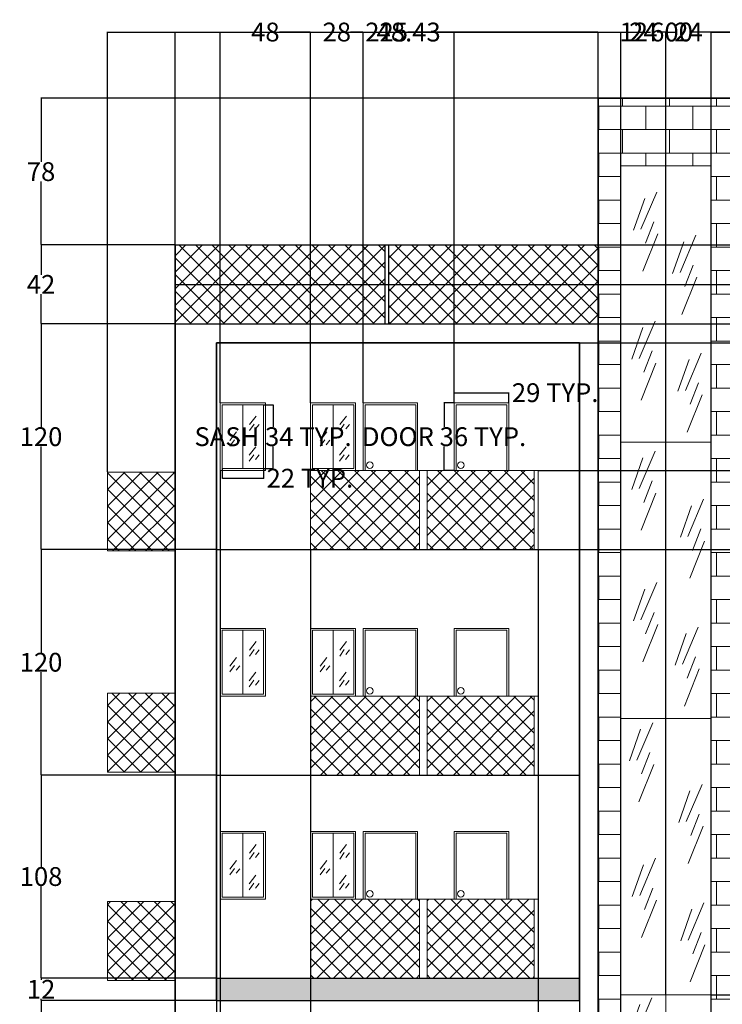
# Model space of a CAD drawing. Units: inches. Extents: x 183 to 891, y 196 to 984.
# Tile 2 of 3: x 192 to 566, y 460 to 984. Entities that reach past the tile are written whole.
import ezdxf

# ---------------------------------------------------------------- set-up
doc = ezdxf.new("R2010")
doc.units = ezdxf.units.IN
doc.header["$MEASUREMENT"] = 0
for name, color, linetype, lineweight in [('A-ANNO-DIMS', 2, 'Continuous', 18), ('A-DOOR', 3, 'Continuous', 20), ('A-FLOR', 7, 'Continuous', 30), ('A-FLOR-PATT', 2, 'Continuous', 13), ('A-GLAZ', 4, 'Continuous', 18), ('A-GLAZ-DETL', 4, 'Continuous', 13), ('A-RAIL', 7, 'Continuous', 20), ('A-RAIL-PATT', 8, 'Continuous', 13), ('A-ROOF', 7, 'Continuous', 25), ('A-WALL', 7, 'Continuous', 35), ('A-WALL-PATT', 251, 'Continuous', 13)]:
    doc.layers.add(name, color=color, linetype=linetype, lineweight=lineweight)
doc.styles.get("Standard").update_dxf_attribs({"font": 'arial.ttf'})
doc.dimstyles.get("Standard").update_dxf_attribs({"dimtxt": 10, "dimasz": 0.18, "dimexe": 0.18, "dimexo": 0.0625, "dimgap": 0.09, "dimtad": 0, "dimtih": 1, "dimtoh": 1, "dimdec": 0, "dimzin": 0, "dimdsep": 46, "dimlunit": 3, "dimtxsty": 'Standard', "dimcen": 0.09, "dimadec": 0, "dimazin": 0, "dimtfac": 1, "dimtdec": 0, "dimtofl": 0, "dimtmove": 0, "dimatfit": 3, "dimfxl": 1, "dimtolj": 1, "dimtzin": 0, "dimarcsym": 0})

# ---------------------------------------------------------------- blocks, each defined once
blk = doc.blocks.new('WIN-SASH-PAIR-22X34')
for p, q in [((11, 34), (11, 0)), ((18.11, 27.96), (14.53, 23.4)), ((16.98, 23.73), (14.53, 20.31)), ((19.74, 23.56), (17.79, 21.12)), ((7.74, 19.54), (4.16, 14.99)), ((6.61, 15.31), (4.16, 11.9)), ((9.37, 15.15), (7.42, 12.71)), ((18.01, 11.64), (14.43, 7.09)), ((16.87, 7.41), (14.43, 4)), ((19.64, 7.25), (17.69, 4.81))]:
    blk.add_line(p, q)
blk.add_lwpolyline([(0, 0), (22, 0), (22, 34), (0, 34)], close=True)
blk = doc.blocks.new('DOOR-BALCONY-ELEV-29')
for p, q in [((0, 0), (0, 36)), ((0, 36), (29, 36)), ((1, 35), (28, 35)), ((1, 0), (1, 35)), ((28, 35), (28, 0)), ((29, 36), (29, 0))]:
    blk.add_line(p, q)
blk.add_circle((3.53, 2.84), 1.74)
blk = doc.blocks.new('GLASS-REFLECTION-ELEV')
for p, q in [((12.39, 42.09), (3.96, 22.28)), ((5.95, 38.63), (0, 21.79)), ((10.9, 26.25), (6.44, 14.86)), ((12.89, 19.81), (4.96, 0))]:
    blk.add_line(p, q)
blk = doc.blocks.new('*D4')
at = {"layer": 'A-ANNO-DIMS', "color": 0, "lineweight": -2, "transparency": 16777216}
for p, q in [((321.66, 778.68), (326.88, 778.68)), ((326.7, 778.5), (326.7, 766.94)), ((326.7, 744.86), (326.7, 756.41)), ((321.66, 744.68), (326.88, 744.68))]:
    blk.add_line(p, q, dxfattribs=at)
at = {"layer": 'A-ANNO-DIMS', "color": 0, "transparency": 16777216}
for points in [[(326.67, 778.5), (326.73, 778.5), (326.7, 778.68)], [(326.67, 744.86), (326.73, 744.86), (326.7, 744.68)]]:
    blk.add_solid(points, dxfattribs=at)
at = {"layer": 'Defpoints', "color": 0, "transparency": 16777216}
for p in [(321.6, 778.68), (326.7, 778.68), (321.6, 744.68)]:
    blk.add_point(p, dxfattribs=at)
at = {"layer": 'A-ANNO-DIMS', "color": 0, "transparency": 16777216, "insert": (326.7, 761.68), "char_height": 10, "attachment_point": 5}
blk.add_mtext('\\A1;SASH 34 TYP.', dxfattribs=at)
blk = doc.blocks.new('*D5')
at = {"layer": 'A-ANNO-DIMS', "color": 0, "lineweight": -2, "transparency": 16777216}
for p, q in [((299.6, 744.61), (299.6, 739.4)), ((321.6, 744.61), (321.6, 739.4)), ((299.78, 739.58), (321.42, 739.58)), ((321.6, 739.58), (321.78, 739.58))]:
    blk.add_line(p, q, dxfattribs=at)
at = {"layer": 'A-ANNO-DIMS', "color": 0, "transparency": 16777216}
for points in [[(299.78, 739.61), (299.78, 739.55), (299.6, 739.58)], [(321.42, 739.61), (321.42, 739.55), (321.6, 739.58)]]:
    blk.add_solid(points, dxfattribs=at)
at = {"layer": 'Defpoints', "color": 0, "transparency": 16777216}
for p in [(299.6, 744.68), (321.6, 744.68), (321.6, 739.58)]:
    blk.add_point(p, dxfattribs=at)
at = {"layer": 'A-ANNO-DIMS', "color": 0, "transparency": 16777216, "insert": (346.29, 739.58), "char_height": 10, "attachment_point": 5}
blk.add_mtext('\\A1;22 TYP.', dxfattribs=at)
blk = doc.blocks.new('*D6')
at = {"layer": 'A-ANNO-DIMS', "color": 0, "lineweight": -2, "transparency": 16777216}
for p, q in [((422.96, 779.68), (417.45, 779.68)), ((417.63, 779.5), (417.63, 766.94)), ((417.63, 743.86), (417.63, 756.41)), ((422.96, 743.68), (417.45, 743.68))]:
    blk.add_line(p, q, dxfattribs=at)
at = {"layer": 'A-ANNO-DIMS', "color": 0, "transparency": 16777216}
for points in [[(417.6, 779.5), (417.66, 779.5), (417.63, 779.68)], [(417.6, 743.86), (417.66, 743.86), (417.63, 743.68)]]:
    blk.add_solid(points, dxfattribs=at)
at = {"layer": 'Defpoints', "color": 0, "transparency": 16777216}
for p in [(417.63, 779.68), (423.03, 779.68), (423.03, 743.68)]:
    blk.add_point(p, dxfattribs=at)
at = {"layer": 'A-ANNO-DIMS', "color": 0, "transparency": 16777216, "insert": (417.63, 761.68), "char_height": 10, "attachment_point": 5}
blk.add_mtext('\\A1;DOOR 36 TYP.', dxfattribs=at)
blk = doc.blocks.new('*D7')
at = {"layer": 'A-ANNO-DIMS', "color": 0, "lineweight": -2, "transparency": 16777216}
for p, q in [((423.03, 779.74), (423.03, 785.26)), ((423.21, 785.08), (451.85, 785.08)), ((452.03, 779.74), (452.03, 785.26)), ((452.03, 785.08), (452.21, 785.08))]:
    blk.add_line(p, q, dxfattribs=at)
at = {"layer": 'A-ANNO-DIMS', "color": 0, "transparency": 16777216}
for points in [[(423.21, 785.11), (423.21, 785.05), (423.03, 785.08)], [(451.85, 785.11), (451.85, 785.05), (452.03, 785.08)]]:
    blk.add_solid(points, dxfattribs=at)
at = {"layer": 'Defpoints', "color": 0, "transparency": 16777216}
for p in [(452.03, 785.08), (423.03, 779.68), (452.03, 779.68)]:
    blk.add_point(p, dxfattribs=at)
at = {"layer": 'A-ANNO-DIMS', "color": 0, "transparency": 16777216, "insert": (476.72, 785.08), "char_height": 10, "attachment_point": 5}
blk.add_mtext('\\A1;29 TYP.', dxfattribs=at)
blk = doc.blocks.new('*D8')
at = {"layer": 'A-ANNO-DIMS', "color": 0, "lineweight": -2, "transparency": 16777216}
for p, q in [((238.6, 742.93), (238.6, 977.12)), ((238.78, 976.94), (527.45, 976.94)), ((838.42, 976.94), (549.75, 976.94)), ((838.6, 743.74), (838.6, 977.12))]:
    blk.add_line(p, q, dxfattribs=at)
at = {"layer": 'A-ANNO-DIMS', "color": 0, "transparency": 16777216}
for points in [[(238.78, 976.97), (238.78, 976.91), (238.6, 976.94)], [(838.42, 976.97), (838.42, 976.91), (838.6, 976.94)]]:
    blk.add_solid(points, dxfattribs=at)
at = {"layer": 'Defpoints', "color": 0, "transparency": 16777216}
for p in [(838.6, 976.94), (238.6, 742.86), (838.6, 743.68)]:
    blk.add_point(p, dxfattribs=at)
at = {"layer": 'A-ANNO-DIMS', "color": 0, "transparency": 16777216, "insert": (538.6, 976.94), "char_height": 10, "attachment_point": 5}
blk.add_mtext('\\A1;600', dxfattribs=at)
blk = doc.blocks.new('*D10')
at = {"layer": 'A-ANNO-DIMS', "color": 0, "lineweight": -2, "transparency": 16777216}
for p, q in [((274.6, 863.74), (274.6, 977.12)), ((274.78, 976.94), (375.84, 976.94)), ((499.42, 976.94), (398.36, 976.94)), ((499.6, 863.74), (499.6, 977.12))]:
    blk.add_line(p, q, dxfattribs=at)
at = {"layer": 'A-ANNO-DIMS', "color": 0, "transparency": 16777216}
for points in [[(274.78, 976.97), (274.78, 976.91), (274.6, 976.94)], [(499.42, 976.97), (499.42, 976.91), (499.6, 976.94)]]:
    blk.add_solid(points, dxfattribs=at)
at = {"layer": 'Defpoints', "color": 0, "transparency": 16777216}
for p in [(499.6, 976.94), (274.6, 863.68), (499.6, 863.68)]:
    blk.add_point(p, dxfattribs=at)
at = {"layer": 'A-ANNO-DIMS', "color": 0, "transparency": 16777216, "insert": (387.1, 976.94), "char_height": 10, "attachment_point": 5}
blk.add_mtext('\\A1;225', dxfattribs=at)
blk = doc.blocks.new('*D27')
at = {"layer": 'A-ANNO-DIMS', "color": 0, "lineweight": -2, "transparency": 16777216}
for p, q in [((296.54, 461.68), (203.15, 461.68)), ((203.33, 461.5), (203.33, 406.87)), ((203.33, 341.86), (203.33, 396.48)), ((274.54, 341.68), (203.15, 341.68))]:
    blk.add_line(p, q, dxfattribs=at)
at = {"layer": 'A-ANNO-DIMS', "color": 0, "transparency": 16777216}
for points in [[(203.3, 461.5), (203.36, 461.5), (203.33, 461.68)], [(203.3, 341.86), (203.36, 341.86), (203.33, 341.68)]]:
    blk.add_solid(points, dxfattribs=at)
at = {"layer": 'Defpoints', "color": 0, "transparency": 16777216}
for p in [(203.33, 461.68), (296.6, 461.68), (274.6, 341.68)]:
    blk.add_point(p, dxfattribs=at)
at = {"layer": 'A-ANNO-DIMS', "color": 0, "transparency": 16777216, "insert": (203.33, 401.68), "char_height": 10, "attachment_point": 5}
blk.add_mtext('\\A1;120', dxfattribs=at)
blk = doc.blocks.new('*D28')
at = {"layer": 'A-ANNO-DIMS', "color": 0, "lineweight": -2, "transparency": 16777216}
for p, q in [((296.54, 473.68), (203.15, 473.68)), ((203.33, 473.5), (203.33, 472.79)), ((296.54, 461.68), (203.15, 461.68)), ((203.33, 461.86), (203.33, 462.56))]:
    blk.add_line(p, q, dxfattribs=at)
at = {"layer": 'A-ANNO-DIMS', "color": 0, "transparency": 16777216}
for points in [[(203.3, 473.5), (203.36, 473.5), (203.33, 473.68)], [(203.3, 461.86), (203.36, 461.86), (203.33, 461.68)]]:
    blk.add_solid(points, dxfattribs=at)
at = {"layer": 'Defpoints', "color": 0, "transparency": 16777216}
for p in [(203.33, 473.68), (296.6, 473.68), (296.6, 461.68)]:
    blk.add_point(p, dxfattribs=at)
at = {"layer": 'A-ANNO-DIMS', "color": 0, "transparency": 16777216, "insert": (203.33, 467.68), "char_height": 10, "attachment_point": 5}
blk.add_mtext('\\A1;12', dxfattribs=at)
blk = doc.blocks.new('*D29')
at = {"layer": 'A-ANNO-DIMS', "color": 0, "lineweight": -2, "transparency": 16777216}
for p, q in [((296.54, 581.68), (203.15, 581.68)), ((203.33, 581.5), (203.33, 532.87)), ((203.33, 473.86), (203.33, 522.48)), ((296.54, 473.68), (203.15, 473.68))]:
    blk.add_line(p, q, dxfattribs=at)
at = {"layer": 'A-ANNO-DIMS', "color": 0, "transparency": 16777216}
for points in [[(203.3, 581.5), (203.36, 581.5), (203.33, 581.68)], [(203.3, 473.86), (203.36, 473.86), (203.33, 473.68)]]:
    blk.add_solid(points, dxfattribs=at)
at = {"layer": 'Defpoints', "color": 0, "transparency": 16777216}
for p in [(203.33, 581.68), (296.6, 581.68), (296.6, 473.68)]:
    blk.add_point(p, dxfattribs=at)
at = {"layer": 'A-ANNO-DIMS', "color": 0, "transparency": 16777216, "insert": (203.33, 527.68), "char_height": 10, "attachment_point": 5}
blk.add_mtext('\\A1;108', dxfattribs=at)
blk = doc.blocks.new('*D30')
at = {"layer": 'A-ANNO-DIMS', "color": 0, "lineweight": -2, "transparency": 16777216}
for p, q in [((296.54, 701.68), (203.15, 701.68)), ((203.33, 701.5), (203.33, 646.87)), ((203.33, 581.86), (203.33, 636.48)), ((296.54, 581.68), (203.15, 581.68))]:
    blk.add_line(p, q, dxfattribs=at)
at = {"layer": 'A-ANNO-DIMS', "color": 0, "transparency": 16777216}
for points in [[(203.3, 701.5), (203.36, 701.5), (203.33, 701.68)], [(203.3, 581.86), (203.36, 581.86), (203.33, 581.68)]]:
    blk.add_solid(points, dxfattribs=at)
at = {"layer": 'Defpoints', "color": 0, "transparency": 16777216}
for p in [(203.33, 701.68), (296.6, 701.68), (296.6, 581.68)]:
    blk.add_point(p, dxfattribs=at)
at = {"layer": 'A-ANNO-DIMS', "color": 0, "transparency": 16777216, "insert": (203.33, 641.68), "char_height": 10, "attachment_point": 5}
blk.add_mtext('\\A1;120', dxfattribs=at)
blk = doc.blocks.new('*D31')
at = {"layer": 'A-ANNO-DIMS', "color": 0, "lineweight": -2, "transparency": 16777216}
for p, q in [((274.54, 821.68), (203.15, 821.68)), ((203.33, 821.5), (203.33, 766.87)), ((203.33, 701.86), (203.33, 756.48)), ((296.54, 701.68), (203.15, 701.68))]:
    blk.add_line(p, q, dxfattribs=at)
at = {"layer": 'A-ANNO-DIMS', "color": 0, "transparency": 16777216}
for points in [[(203.3, 821.5), (203.36, 821.5), (203.33, 821.68)], [(203.3, 701.86), (203.36, 701.86), (203.33, 701.68)]]:
    blk.add_solid(points, dxfattribs=at)
at = {"layer": 'Defpoints', "color": 0, "transparency": 16777216}
for p in [(203.33, 821.68), (274.6, 821.68), (296.6, 701.68)]:
    blk.add_point(p, dxfattribs=at)
at = {"layer": 'A-ANNO-DIMS', "color": 0, "transparency": 16777216, "insert": (203.33, 761.68), "char_height": 10, "attachment_point": 5}
blk.add_mtext('\\A1;120', dxfattribs=at)
blk = doc.blocks.new('*D32')
at = {"layer": 'A-ANNO-DIMS', "color": 0, "lineweight": -2, "transparency": 16777216}
for p, q in [((274.54, 863.68), (203.15, 863.68)), ((203.33, 863.5), (203.33, 847.79)), ((203.33, 821.86), (203.33, 837.56)), ((274.54, 821.68), (203.15, 821.68))]:
    blk.add_line(p, q, dxfattribs=at)
at = {"layer": 'A-ANNO-DIMS', "color": 0, "transparency": 16777216}
for points in [[(203.3, 863.5), (203.36, 863.5), (203.33, 863.68)], [(203.3, 821.86), (203.36, 821.86), (203.33, 821.68)]]:
    blk.add_solid(points, dxfattribs=at)
at = {"layer": 'Defpoints', "color": 0, "transparency": 16777216}
for p in [(203.33, 863.68), (274.6, 863.68), (274.6, 821.68)]:
    blk.add_point(p, dxfattribs=at)
at = {"layer": 'A-ANNO-DIMS', "color": 0, "transparency": 16777216, "insert": (203.33, 842.68), "char_height": 10, "attachment_point": 5}
blk.add_mtext('\\A1;42', dxfattribs=at)
blk = doc.blocks.new('*D33')
at = {"layer": 'A-ANNO-DIMS', "color": 0, "lineweight": -2, "transparency": 16777216}
for p, q in [((499.54, 941.68), (203.15, 941.68)), ((203.33, 941.5), (203.33, 907.87)), ((203.33, 863.86), (203.33, 897.48)), ((274.54, 863.68), (203.15, 863.68))]:
    blk.add_line(p, q, dxfattribs=at)
at = {"layer": 'A-ANNO-DIMS', "color": 0, "transparency": 16777216}
for points in [[(203.3, 941.5), (203.36, 941.5), (203.33, 941.68)], [(203.3, 863.86), (203.36, 863.86), (203.33, 863.68)]]:
    blk.add_solid(points, dxfattribs=at)
at = {"layer": 'Defpoints', "color": 0, "transparency": 16777216}
for p in [(203.33, 941.68), (499.6, 941.68), (274.6, 863.68)]:
    blk.add_point(p, dxfattribs=at)
at = {"layer": 'A-ANNO-DIMS', "color": 0, "transparency": 16777216, "insert": (203.33, 902.68), "char_height": 10, "attachment_point": 5}
blk.add_mtext('\\A1;78', dxfattribs=at)
blk = doc.blocks.new('*D34')
at = {"layer": 'A-ANNO-DIMS', "color": 0, "lineweight": -2, "transparency": 16777216}
for p, q in [((511.6, 464.74), (511.6, 977.12)), ((511.78, 976.94), (516.28, 976.94)), ((535.42, 976.94), (530.92, 976.94)), ((535.6, 464.74), (535.6, 977.12))]:
    blk.add_line(p, q, dxfattribs=at)
at = {"layer": 'A-ANNO-DIMS', "color": 0, "transparency": 16777216}
for points in [[(511.78, 976.97), (511.78, 976.91), (511.6, 976.94)], [(535.42, 976.97), (535.42, 976.91), (535.6, 976.94)]]:
    blk.add_solid(points, dxfattribs=at)
at = {"layer": 'Defpoints', "color": 0, "transparency": 16777216}
for p in [(535.6, 976.94), (511.6, 464.68), (535.6, 464.68)]:
    blk.add_point(p, dxfattribs=at)
at = {"layer": 'A-ANNO-DIMS', "color": 0, "transparency": 16777216, "insert": (523.6, 976.94), "char_height": 10, "attachment_point": 5}
blk.add_mtext('\\A1;24', dxfattribs=at)
blk = doc.blocks.new('*D35')
at = {"layer": 'A-ANNO-DIMS', "color": 0, "lineweight": -2, "transparency": 16777216}
for p, q in [((535.6, 464.74), (535.6, 977.12)), ((535.78, 976.94), (540.28, 976.94)), ((559.42, 976.94), (554.92, 976.94)), ((559.6, 464.74), (559.6, 977.12))]:
    blk.add_line(p, q, dxfattribs=at)
at = {"layer": 'A-ANNO-DIMS', "color": 0, "transparency": 16777216}
for points in [[(535.78, 976.97), (535.78, 976.91), (535.6, 976.94)], [(559.42, 976.97), (559.42, 976.91), (559.6, 976.94)]]:
    blk.add_solid(points, dxfattribs=at)
at = {"layer": 'Defpoints', "color": 0, "transparency": 16777216}
for p in [(559.6, 976.94), (535.6, 464.68), (559.6, 464.68)]:
    blk.add_point(p, dxfattribs=at)
at = {"layer": 'A-ANNO-DIMS', "color": 0, "transparency": 16777216, "insert": (547.6, 976.94), "char_height": 10, "attachment_point": 5}
blk.add_mtext('\\A1;24', dxfattribs=at)
blk = doc.blocks.new('*D36')
at = {"layer": 'A-ANNO-DIMS', "color": 0, "lineweight": -2, "transparency": 16777216}
for p, q in [((499.6, 237.57), (499.6, 977.12)), ((499.78, 976.94), (511.42, 976.94)), ((511.6, 317.74), (511.6, 977.12)), ((511.6, 976.94), (511.78, 976.94))]:
    blk.add_line(p, q, dxfattribs=at)
at = {"layer": 'A-ANNO-DIMS', "color": 0, "transparency": 16777216}
for points in [[(499.78, 976.97), (499.78, 976.91), (499.6, 976.94)], [(511.42, 976.97), (511.42, 976.91), (511.6, 976.94)]]:
    blk.add_solid(points, dxfattribs=at)
at = {"layer": 'Defpoints', "color": 0, "transparency": 16777216}
for p in [(511.6, 976.94), (511.6, 317.68), (499.6, 237.51)]:
    blk.add_point(p, dxfattribs=at)
at = {"layer": 'A-ANNO-DIMS', "color": 0, "transparency": 16777216, "insert": (518.51, 976.94), "char_height": 10, "attachment_point": 5}
blk.add_mtext('\\A1;12', dxfattribs=at)
blk = doc.blocks.new('*D37')
at = {"layer": 'A-ANNO-DIMS', "color": 0, "lineweight": -2, "transparency": 16777216}
for p, q in [((559.6, 317.74), (559.6, 977.12)), ((559.78, 976.94), (571.42, 976.94)), ((571.6, 237.57), (571.6, 977.12)), ((571.6, 976.94), (571.78, 976.94))]:
    blk.add_line(p, q, dxfattribs=at)
at = {"layer": 'A-ANNO-DIMS', "color": 0, "transparency": 16777216}
for points in [[(559.78, 976.97), (559.78, 976.91), (559.6, 976.94)], [(571.42, 976.97), (571.42, 976.91), (571.6, 976.94)]]:
    blk.add_solid(points, dxfattribs=at)
at = {"layer": 'Defpoints', "color": 0, "transparency": 16777216}
for p in [(571.6, 976.94), (559.6, 317.68), (571.6, 237.51)]:
    blk.add_point(p, dxfattribs=at)
at = {"layer": 'A-ANNO-DIMS', "color": 0, "transparency": 16777216, "insert": (578.51, 976.94), "char_height": 10, "attachment_point": 5}
blk.add_mtext('\\A1;12', dxfattribs=at)
blk = doc.blocks.new('*D39')
at = {"layer": 'A-ANNO-DIMS', "color": 0, "lineweight": -2, "transparency": 16777216}
for p, q in [((559.66, 464.68), (874.04, 464.68)), ((873.86, 464.5), (873.86, 396.29)), ((873.86, 317.86), (873.86, 386.06)), ((559.66, 317.68), (874.04, 317.68))]:
    blk.add_line(p, q, dxfattribs=at)
at = {"layer": 'A-ANNO-DIMS', "color": 0, "transparency": 16777216}
for points in [[(873.83, 464.5), (873.89, 464.5), (873.86, 464.68)], [(873.83, 317.86), (873.89, 317.86), (873.86, 317.68)]]:
    blk.add_solid(points, dxfattribs=at)
at = {"layer": 'Defpoints', "color": 0, "transparency": 16777216}
for p in [(559.6, 464.68), (873.86, 464.68), (559.6, 317.68)]:
    blk.add_point(p, dxfattribs=at)
at = {"layer": 'A-ANNO-DIMS', "color": 0, "transparency": 16777216, "insert": (873.86, 391.18), "char_height": 10, "attachment_point": 5}
blk.add_mtext('\\A1;147', dxfattribs=at)
blk = doc.blocks.new('*D40')
at = {"layer": 'A-ANNO-DIMS', "color": 0, "lineweight": -2, "transparency": 16777216}
for p, q in [((274.6, 742.8), (274.6, 202.06)), ((298.6, 743.61), (298.6, 202.06)), ((274.78, 202.24), (279.28, 202.24)), ((298.42, 202.24), (293.92, 202.24))]:
    blk.add_line(p, q, dxfattribs=at)
at = {"layer": 'A-ANNO-DIMS', "color": 0, "transparency": 16777216}
for points in [[(274.78, 202.27), (274.78, 202.21), (274.6, 202.24)], [(298.42, 202.27), (298.42, 202.21), (298.6, 202.24)]]:
    blk.add_solid(points, dxfattribs=at)
at = {"layer": 'Defpoints', "color": 0, "transparency": 16777216}
for p in [(274.6, 742.86), (298.6, 743.68), (298.6, 202.24)]:
    blk.add_point(p, dxfattribs=at)
at = {"layer": 'A-ANNO-DIMS', "color": 0, "transparency": 16777216, "insert": (286.6, 202.24), "char_height": 10, "attachment_point": 5}
blk.add_mtext('\\A1;24', dxfattribs=at)
blk = doc.blocks.new('*D41')
at = {"layer": 'A-ANNO-DIMS', "color": 0, "lineweight": -2, "transparency": 16777216}
for p, q in [((298.6, 779.74), (298.6, 977.12)), ((298.78, 976.94), (315.14, 976.94)), ((346.42, 976.94), (330.06, 976.94)), ((346.6, 779.74), (346.6, 977.12))]:
    blk.add_line(p, q, dxfattribs=at)
at = {"layer": 'A-ANNO-DIMS', "color": 0, "transparency": 16777216}
for points in [[(298.78, 976.97), (298.78, 976.91), (298.6, 976.94)], [(346.42, 976.97), (346.42, 976.91), (346.6, 976.94)]]:
    blk.add_solid(points, dxfattribs=at)
at = {"layer": 'Defpoints', "color": 0, "transparency": 16777216}
for p in [(346.6, 976.94), (298.6, 779.68), (346.6, 779.68)]:
    blk.add_point(p, dxfattribs=at)
at = {"layer": 'A-ANNO-DIMS', "color": 0, "transparency": 16777216, "insert": (322.6, 976.94), "char_height": 10, "attachment_point": 5}
blk.add_mtext('\\A1;48', dxfattribs=at)
blk = doc.blocks.new('*D42')
at = {"layer": 'A-ANNO-DIMS', "color": 0, "lineweight": -2, "transparency": 16777216}
for p, q in [((346.6, 779.74), (346.6, 977.12)), ((346.78, 976.94), (353.25, 976.94)), ((374.42, 976.94), (367.95, 976.94)), ((374.6, 779.74), (374.6, 977.12))]:
    blk.add_line(p, q, dxfattribs=at)
at = {"layer": 'A-ANNO-DIMS', "color": 0, "transparency": 16777216}
for points in [[(346.78, 976.97), (346.78, 976.91), (346.6, 976.94)], [(374.42, 976.97), (374.42, 976.91), (374.6, 976.94)]]:
    blk.add_solid(points, dxfattribs=at)
at = {"layer": 'Defpoints', "color": 0, "transparency": 16777216}
for p in [(374.6, 976.94), (346.6, 779.68), (374.6, 779.68)]:
    blk.add_point(p, dxfattribs=at)
at = {"layer": 'A-ANNO-DIMS', "color": 0, "transparency": 16777216, "insert": (360.6, 976.94), "char_height": 10, "attachment_point": 5}
blk.add_mtext('\\A1;28', dxfattribs=at)
blk = doc.blocks.new('*D43')
at = {"layer": 'A-ANNO-DIMS', "color": 0, "lineweight": -2, "transparency": 16777216}
for p, q in [((374.6, 779.74), (374.6, 977.12)), ((374.78, 976.94), (381.65, 976.94)), ((422.85, 976.94), (415.98, 976.94)), ((423.03, 779.74), (423.03, 977.12))]:
    blk.add_line(p, q, dxfattribs=at)
at = {"layer": 'A-ANNO-DIMS', "color": 0, "transparency": 16777216}
for points in [[(374.78, 976.97), (374.78, 976.91), (374.6, 976.94)], [(422.85, 976.97), (422.85, 976.91), (423.03, 976.94)]]:
    blk.add_solid(points, dxfattribs=at)
at = {"layer": 'Defpoints', "color": 0, "transparency": 16777216}
for p in [(423.03, 976.94), (374.6, 779.68), (423.03, 779.68)]:
    blk.add_point(p, dxfattribs=at)
at = {"layer": 'A-ANNO-DIMS', "color": 0, "transparency": 16777216, "insert": (398.81, 976.94), "char_height": 10, "attachment_point": 5}
blk.add_mtext('\\A1;48.43', dxfattribs=at)
blk = doc.blocks.new('*D44')
at = {"layer": 'A-ANNO-DIMS', "color": 0, "lineweight": -2, "transparency": 16777216}
for p, q in [((346.6, 701.61), (346.6, 202.06)), ((467.6, 701.61), (467.6, 202.06)), ((346.78, 202.24), (397.4, 202.24)), ((467.42, 202.24), (416.8, 202.24))]:
    blk.add_line(p, q, dxfattribs=at)
at = {"layer": 'A-ANNO-DIMS', "color": 0, "transparency": 16777216}
for points in [[(346.78, 202.27), (346.78, 202.21), (346.6, 202.24)], [(467.42, 202.27), (467.42, 202.21), (467.6, 202.24)]]:
    blk.add_solid(points, dxfattribs=at)
at = {"layer": 'Defpoints', "color": 0, "transparency": 16777216}
for p in [(346.6, 701.68), (467.6, 701.68), (467.6, 202.24)]:
    blk.add_point(p, dxfattribs=at)
at = {"layer": 'A-ANNO-DIMS', "color": 0, "transparency": 16777216, "insert": (407.1, 202.24), "char_height": 10, "attachment_point": 5}
blk.add_mtext('\\A1;121', dxfattribs=at)
blk = doc.blocks.new('*D45')
at = {"layer": 'A-ANNO-DIMS', "color": 0, "lineweight": -2, "transparency": 16777216}
for p, q in [((467.66, 743.68), (874.04, 743.68)), ((873.86, 743.5), (873.86, 727.79)), ((873.86, 701.86), (873.86, 717.56)), ((467.66, 701.68), (874.04, 701.68))]:
    blk.add_line(p, q, dxfattribs=at)
at = {"layer": 'A-ANNO-DIMS', "color": 0, "transparency": 16777216}
for points in [[(873.83, 743.5), (873.89, 743.5), (873.86, 743.68)], [(873.83, 701.86), (873.89, 701.86), (873.86, 701.68)]]:
    blk.add_solid(points, dxfattribs=at)
at = {"layer": 'Defpoints', "color": 0, "transparency": 16777216}
for p in [(467.6, 743.68), (873.86, 743.68), (467.6, 701.68)]:
    blk.add_point(p, dxfattribs=at)
at = {"layer": 'A-ANNO-DIMS', "color": 0, "transparency": 16777216, "insert": (873.86, 722.68), "char_height": 10, "attachment_point": 5}
blk.add_mtext('\\A1;42', dxfattribs=at)
blk = doc.blocks.new('*D46')
at = {"layer": 'A-ANNO-DIMS', "color": 0, "lineweight": -2, "transparency": 16777216}
for p, q in [((274.6, 821.61), (274.6, 202.06)), ((296.6, 811.61), (296.6, 202.06)), ((274.78, 202.24), (278.31, 202.24)), ((296.42, 202.24), (292.89, 202.24))]:
    blk.add_line(p, q, dxfattribs=at)
at = {"layer": 'A-ANNO-DIMS', "color": 0, "transparency": 16777216}
for points in [[(274.78, 202.27), (274.78, 202.21), (274.6, 202.24)], [(296.42, 202.27), (296.42, 202.21), (296.6, 202.24)]]:
    blk.add_solid(points, dxfattribs=at)
at = {"layer": 'Defpoints', "color": 0, "transparency": 16777216}
for p in [(274.6, 821.68), (296.6, 811.68), (296.6, 202.24)]:
    blk.add_point(p, dxfattribs=at)
at = {"layer": 'A-ANNO-DIMS', "color": 0, "transparency": 16777216, "insert": (285.6, 202.24), "char_height": 10, "attachment_point": 5}
blk.add_mtext('\\A1;22', dxfattribs=at)
blk = doc.blocks.new('*D47')
at = {"layer": 'A-ANNO-DIMS', "color": 0, "lineweight": -2, "transparency": 16777216}
for p, q in [((499.6, 821.61), (499.6, 202.06)), ((489.6, 811.61), (489.6, 202.06)), ((489.78, 202.24), (499.42, 202.24)), ((499.6, 202.24), (499.78, 202.24))]:
    blk.add_line(p, q, dxfattribs=at)
at = {"layer": 'A-ANNO-DIMS', "color": 0, "transparency": 16777216}
for points in [[(489.78, 202.27), (489.78, 202.21), (489.6, 202.24)], [(499.42, 202.27), (499.42, 202.21), (499.6, 202.24)]]:
    blk.add_solid(points, dxfattribs=at)
at = {"layer": 'Defpoints', "color": 0, "transparency": 16777216}
for p in [(499.6, 821.68), (489.6, 811.68), (499.6, 202.24)]:
    blk.add_point(p, dxfattribs=at)
at = {"layer": 'A-ANNO-DIMS', "color": 0, "transparency": 16777216, "insert": (506.54, 202.24), "char_height": 10, "attachment_point": 5}
blk.add_mtext('\\A1;10', dxfattribs=at)
blk = doc.blocks.new('*D48')
at = {"layer": 'A-ANNO-DIMS', "color": 0, "lineweight": -2, "transparency": 16777216}
for p, q in [((499.66, 821.68), (874.04, 821.68)), ((873.86, 821.68), (873.86, 821.86)), ((873.86, 821.86), (874.04, 821.86)), ((873.86, 811.86), (873.86, 821.5)), ((489.66, 811.68), (874.04, 811.68))]:
    blk.add_line(p, q, dxfattribs=at)
at = {"layer": 'A-ANNO-DIMS', "color": 0, "transparency": 16777216}
for points in [[(873.83, 821.5), (873.89, 821.5), (873.86, 821.68)], [(873.83, 811.86), (873.89, 811.86), (873.86, 811.68)]]:
    blk.add_solid(points, dxfattribs=at)
at = {"layer": 'Defpoints', "color": 0, "transparency": 16777216}
for p in [(499.6, 821.68), (873.86, 821.68), (489.6, 811.68)]:
    blk.add_point(p, dxfattribs=at)
at = {"layer": 'A-ANNO-DIMS', "color": 0, "transparency": 16777216, "insert": (880.81, 821.86), "char_height": 10, "attachment_point": 5}
blk.add_mtext('\\A1;10', dxfattribs=at)
blk = doc.blocks.new('*D49')
at = {"layer": 'A-ANNO-DIMS', "color": 0, "lineweight": -2, "transparency": 16777216}
for p, q in [((499.66, 863.68), (874.04, 863.68)), ((873.86, 863.5), (873.86, 858.29)), ((873.86, 842.86), (873.86, 848.06)), ((499.66, 842.68), (874.04, 842.68))]:
    blk.add_line(p, q, dxfattribs=at)
at = {"layer": 'A-ANNO-DIMS', "color": 0, "transparency": 16777216}
for points in [[(873.83, 863.5), (873.89, 863.5), (873.86, 863.68)], [(873.83, 842.86), (873.89, 842.86), (873.86, 842.68)]]:
    blk.add_solid(points, dxfattribs=at)
at = {"layer": 'Defpoints', "color": 0, "transparency": 16777216}
for p in [(499.6, 863.68), (873.86, 863.68), (499.6, 842.68)]:
    blk.add_point(p, dxfattribs=at)
at = {"layer": 'A-ANNO-DIMS', "color": 0, "transparency": 16777216, "insert": (873.86, 853.18), "char_height": 10, "attachment_point": 5}
blk.add_mtext('\\A1;21', dxfattribs=at)

msp = doc.modelspace()

# ---------------------------------------------------------------- hatches: boundary and pattern name
at = {"layer": 'A-FLOR-PATT'}
h = msp.add_hatch(color=256, dxfattribs=at)
h.dxf.hatch_style = 1
h.paths.add_polyline_path([(489.599, 473.6754), (296.599, 473.6754), (296.599, 461.6754), (489.599, 461.6754)])
h.paths.add_polyline_path([(780.599, 473.6754), (581.599, 473.6754), (581.599, 461.6754), (780.599, 461.6754)])
at = {"layer": 'A-RAIL-PATT'}
h = msp.add_hatch(dxfattribs=at)
h.set_pattern_fill('ANSI37', color=256, scale=50)
h.paths.add_polyline_path([(386.099, 842.6754), (274.599, 842.6754), (274.599, 821.6754), (386.099, 821.6754)])
h.paths.add_polyline_path([(386.099, 863.6754), (274.599, 863.6754), (274.599, 842.6754), (386.099, 842.6754)])
h.paths.add_polyline_path([(499.599, 863.6754), (388.099, 863.6754), (388.099, 842.6754), (499.599, 842.6754)])
h.paths.add_polyline_path([(499.599, 842.6754), (388.099, 842.6754), (388.099, 821.6754), (499.599, 821.6754)])
h.paths.add_polyline_path([(686.099, 863.6754), (571.599, 863.6754), (571.599, 842.6754), (686.099, 842.6754)])
h.paths.add_polyline_path([(686.099, 842.6754), (571.599, 842.6754), (571.599, 821.6754), (634.599, 821.6754), (686.099, 821.6754)])
h.paths.add_polyline_path([(802.599, 863.6754), (688.099, 863.6754), (688.099, 842.6754), (802.599, 842.6754)])
h.paths.add_polyline_path([(802.599, 842.6754), (688.099, 842.6754), (688.099, 821.6754), (802.599, 821.6754)])
h = msp.add_hatch(dxfattribs=at)
h.set_pattern_fill('ANSI37', color=256, scale=50)
h.paths.add_polyline_path([(404.599, 743.6754), (346.599, 743.6754), (346.599, 701.6754), (404.599, 701.6754)])
h.paths.add_polyline_path([(465.599, 743.6754), (408.599, 743.6754), (408.599, 701.6754), (465.599, 701.6754)])
h.paths.add_polyline_path([(668.2227, 743.6754), (611.2227, 743.6754), (611.2227, 701.6754), (668.2227, 701.6754)])
h.paths.add_polyline_path([(730.2227, 743.6754), (706.2227, 743.6754), (672.2227, 743.6754), (672.2227, 701.6754), (730.2227, 701.6754)])
h.paths.add_polyline_path([(838.599, 743.6754), (802.599, 743.6754), (802.599, 701.6754), (838.599, 701.6754)])
h.paths.add_polyline_path([(274.599, 742.8641), (238.599, 742.8641), (238.599, 700.8641), (274.599, 700.8641)])
h.paths.add_polyline_path([(274.599, 625.2404), (238.599, 625.2404), (238.599, 583.2404), (274.599, 583.2404)])
h.paths.add_polyline_path([(404.599, 623.6754), (346.599, 623.6754), (346.599, 581.6754), (404.599, 581.6754)])
h.paths.add_polyline_path([(465.599, 623.6754), (408.599, 623.6754), (408.599, 581.6754), (465.599, 581.6754)])
h.paths.add_polyline_path([(668.2227, 623.6754), (611.2227, 623.6754), (611.2227, 581.6754), (668.2227, 581.6754)])
h.paths.add_polyline_path([(730.2227, 623.6754), (672.2227, 623.6754), (672.2227, 581.6754), (730.2227, 581.6754)])
h.paths.add_polyline_path([(838.599, 625.42), (802.599, 625.42), (802.599, 583.42), (838.599, 583.42)])
h.paths.add_polyline_path([(404.599, 515.6754), (346.599, 515.6754), (346.599, 473.6754), (404.599, 473.6754)])
h.paths.add_polyline_path([(465.599, 515.6754), (408.599, 515.6754), (408.599, 473.6754), (465.599, 473.6754)])
h.paths.add_polyline_path([(668.2227, 515.6754), (611.2227, 515.6754), (611.2227, 473.6754), (668.2227, 473.6754)])
h.paths.add_polyline_path([(730.2227, 515.6754), (706.2227, 515.6754), (672.2227, 515.6754), (672.2227, 473.6754), (730.2227, 473.6754)])
h.paths.add_polyline_path([(838.599, 514.8979), (802.599, 514.8979), (802.599, 472.8979), (838.599, 472.8979)])
h.paths.add_polyline_path([(668.2227, 383.6754), (611.2227, 383.6754), (611.2227, 341.6754), (668.2227, 341.6754)])
h.paths.add_polyline_path([(609.2227, 383.6754), (571.599, 383.6754), (571.599, 341.6754), (601.2227, 341.6754), (609.2227, 341.6754)])
h.paths.add_polyline_path([(730.2227, 383.6754), (672.2227, 383.6754), (672.2227, 341.6754), (730.2227, 341.6754)])
h.paths.add_polyline_path([(838.599, 383.6754), (802.599, 383.6754), (802.599, 341.6754), (838.599, 341.6754)])
h.paths.add_polyline_path([(499.599, 383.6754), (467.599, 383.6754), (467.599, 341.6754), (499.599, 341.6754)])
h.paths.add_polyline_path([(465.599, 383.6754), (408.599, 383.6754), (408.599, 341.6754), (465.599, 341.6754)])
h.paths.add_polyline_path([(404.599, 383.6754), (346.599, 383.6754), (346.599, 341.6754), (404.599, 341.6754)])
h.paths.add_polyline_path([(274.599, 383.6754), (238.599, 383.6754), (238.599, 341.6754), (274.599, 341.6754)])
h.paths.add_polyline_path([(274.599, 514.3451), (238.599, 514.3451), (238.599, 472.3451), (274.599, 472.3451)])
at = {"layer": 'A-WALL-PATT'}
h = msp.add_hatch(dxfattribs=at)
h.set_pattern_fill('BRICK', color=256, scale=50)
h.paths.add_polyline_path([(571.599, 341.6754), (571.599, 821.6754), (571.599, 905.6754), (571.599, 941.6754), (499.599, 941.6754), (499.599, 905.6754), (499.599, 821.6754), (499.599, 341.6754), (499.599, 237.5076), (571.599, 237.5076)])
h.paths.add_polyline_path([(511.599, 317.6754), (511.599, 905.6754), (559.599, 905.6754), (559.599, 317.6754)], flags=16)

# ---------------------------------------------------------------- linework, layer by layer
at = {"layer": 'A-FLOR'}
for p, q in [((296.599, 701.6754), (489.599, 701.6754)), ((296.599, 581.6754), (489.599, 581.6754)), ((296.599, 473.6754), (489.599, 473.6754)), ((296.599, 461.6754), (489.599, 461.6754))]:
    msp.add_line(p, q, dxfattribs=at)
at = {"layer": 'A-GLAZ'}
for p, q in [((511.599, 821.6754), (511.599, 905.6754)), ((535.599, 905.6754), (535.599, 317.6754)), ((535.599, 611.6754), (535.599, 905.6754)), ((559.599, 905.6754), (559.599, 821.6754)), ((559.599, 758.6754), (511.599, 758.6754)), ((535.599, 758.6754), (559.599, 758.6754)), ((298.599, 743.6754), (322.599, 743.6754)), ((298.599, 623.6754), (322.599, 623.6754)), ((511.599, 611.6754), (559.599, 611.6754)), ((535.599, 611.6754), (535.599, 317.6754)), ((298.599, 515.6754), (322.599, 515.6754)), ((535.599, 464.6754), (511.599, 464.6754)), ((535.599, 464.6754), (559.599, 464.6754))]:
    msp.add_line(p, q, dxfattribs=at)
for points in [[(511.599, 905.6754), (559.599, 905.6754), (559.599, 317.6754), (511.599, 317.6754)], [(298.599, 743.6754), (322.599, 743.6754), (322.599, 779.6754), (298.599, 779.6754)], [(346.599, 743.6754), (370.599, 743.6754), (370.599, 779.6754), (346.599, 779.6754)], [(298.599, 623.6754), (322.599, 623.6754), (322.599, 659.6754), (298.599, 659.6754)], [(346.599, 623.6754), (370.599, 623.6754), (370.599, 659.6754), (346.599, 659.6754)], [(298.599, 515.6754), (322.599, 515.6754), (322.599, 551.6754), (298.599, 551.6754)], [(346.599, 515.6754), (370.599, 515.6754), (370.599, 551.6754), (346.599, 551.6754)]]:
    msp.add_lwpolyline(points, close=True, dxfattribs=at)
at = {"layer": 'A-RAIL'}
for p, q in [((238.599, 700.8641), (238.599, 742.8641)), ((238.599, 742.8641), (274.599, 742.8641)), ((346.599, 743.6754), (346.599, 701.6754)), ((346.599, 743.6754), (467.599, 743.6754)), ((404.599, 743.4954), (404.599, 701.6754)), ((408.599, 743.4954), (408.599, 701.6754)), ((465.599, 701.6754), (465.599, 743.6754)), ((467.599, 701.6754), (467.599, 743.6754)), ((274.599, 700.8641), (238.599, 700.8641)), ((238.599, 583.2404), (238.599, 625.2404)), ((238.599, 625.2404), (274.599, 625.2404)), ((346.599, 623.6754), (346.599, 581.6754)), ((346.599, 623.6754), (467.599, 623.6754)), ((404.599, 623.4954), (404.599, 581.6754)), ((408.599, 623.4954), (408.599, 581.6754)), ((465.599, 581.6754), (465.599, 623.6754)), ((467.599, 581.6754), (467.599, 623.6754)), ((274.599, 583.2404), (238.599, 583.2404)), ((238.599, 472.3451), (238.599, 514.3451)), ((238.599, 514.3451), (274.599, 514.3451)), ((346.599, 515.6754), (346.599, 473.6754)), ((346.599, 515.6754), (467.599, 515.6754)), ((404.599, 515.4954), (404.599, 473.6754)), ((408.599, 515.4954), (408.599, 473.6754)), ((465.599, 473.6754), (465.599, 515.6754)), ((467.599, 473.6754), (467.599, 515.6754)), ((274.599, 472.3451), (238.599, 472.3451))]:
    msp.add_line(p, q, dxfattribs=at)
at = {"layer": 'A-ROOF'}
for p, q in [((274.599, 863.6754), (499.599, 863.6754)), ((274.599, 863.6754), (499.599, 863.6754)), ((386.099, 863.6754), (386.099, 821.6754)), ((388.099, 863.6754), (388.099, 821.6754)), ((274.599, 842.6754), (499.599, 842.6754)), ((274.599, 821.6754), (499.599, 821.6754))]:
    msp.add_line(p, q, dxfattribs=at)
at = {"layer": 'A-WALL'}
for p, q in [((499.599, 905.6754), (499.599, 941.6754)), ((499.599, 941.6754), (571.599, 941.6754)), ((499.599, 821.6754), (499.599, 905.6754)), ((274.599, 863.6754), (274.599, 237.5076)), ((499.599, 821.6754), (499.599, 341.6754)), ((296.599, 811.6754), (296.599, 461.6754)), ((296.599, 811.6754), (489.599, 811.6754)), ((489.599, 811.6754), (489.599, 461.6754))]:
    msp.add_line(p, q, dxfattribs=at)

# ---------------------------------------------------------------- block references
at = {"layer": 'A-DOOR'}
for p in [(374.599, 743.675), (423.0255, 743.675), (374.599, 623.675), (423.0255, 623.675), (374.599, 515.675), (423.0255, 515.675)]:
    msp.add_blockref('DOOR-BALCONY-ELEV-29', p, dxfattribs=at)
at = {"layer": 'A-GLAZ'}
for p in [(299.599, 744.675), (347.599, 744.675), (299.599, 624.675), (347.599, 624.675), (299.599, 516.675), (347.599, 516.675)]:
    msp.add_blockref('WIN-SASH-PAIR-22X34', p, dxfattribs=at)
at = {"layer": 'A-GLAZ-DETL'}
for p in [(518.379, 849.727), (539.1885, 826.7296), (517.4331, 781.0498), (542.0262, 764.038), (517.4398, 711.8576), (543.294, 686.3399), (518.3856, 641.9202), (540.4563, 618.2927), (516.2264, 567.3873), (542.459, 534.6239), (517.7398, 495.3077), (543.468, 471.6172), (515.7286, 421.0131)]:
    msp.add_blockref('GLASS-REFLECTION-ELEV', p, dxfattribs=at)

# ---------------------------------------------------------------- dimensions: what is measured, and where the dimension line sits
at = {"layer": 'A-ANNO-DIMS'}
for base, p1, p2, override, picture, middle in [((838.599, 976.9404), (238.599, 742.8641), (838.599, 743.6754), {"dimdec": 0, "dimlfac": 1, "dimrnd": 0, "dimzin": 0, "dimdsep": 46, "dimlunit": 2}, '*D8', (538.599, 976.9404)), ((499.599, 976.9404), (274.599, 863.6754), (499.599, 863.6754), {"dimdec": 0, "dimlfac": 1, "dimrnd": 0, "dimzin": 0, "dimdsep": 46, "dimlunit": 2}, '*D10', (387.099, 976.9404)), ((346.599, 976.9404), (298.599, 779.6754), (346.599, 779.6754), {"dimdec": 0, "dimlfac": 1, "dimrnd": 0, "dimzin": 0, "dimdsep": 46, "dimlunit": 2}, '*D41', (322.599, 976.9404)), ((374.599, 976.9404), (346.599, 779.6754), (374.599, 779.6754), {"dimdec": 0, "dimlfac": 1, "dimrnd": 0, "dimzin": 0, "dimdsep": 46, "dimlunit": 2}, '*D42', (360.599, 976.9404)), ((423.0255, 976.9404), (374.599, 779.6754), (423.0255, 779.6754), {"dimdec": 2, "dimlfac": 1, "dimrnd": 0, "dimzin": 0, "dimdsep": 46, "dimlunit": 2}, '*D43', (398.8122, 976.9404)), ((511.599, 976.9404), (499.599, 237.5076), (511.599, 317.6754), {"dimdec": 0, "dimlfac": 1, "dimrnd": 0, "dimzin": 0, "dimdsep": 46, "dimlunit": 2}, '*D36', (518.5095, 976.9404)), ((535.599, 976.9404), (511.599, 464.6754), (535.599, 464.6754), {"dimdec": 0, "dimlfac": 1, "dimrnd": 0, "dimzin": 0, "dimdsep": 46, "dimlunit": 2}, '*D34', (523.599, 976.9404)), ((559.599, 976.9404), (535.599, 464.6754), (559.599, 464.6754), {"dimdec": 0, "dimlfac": 1, "dimrnd": 0, "dimzin": 0, "dimdsep": 46, "dimlunit": 2}, '*D35', (547.599, 976.9404)), ((571.599, 976.9404), (559.599, 317.6754), (571.599, 237.5076), {"dimdec": 0, "dimlfac": 1, "dimrnd": 0, "dimzin": 0, "dimdsep": 46, "dimlunit": 2}, '*D37', (578.5095, 976.9404)), ((296.599, 202.2426), (274.599, 821.6754), (296.599, 811.6754), {"dimdec": 0, "dimlfac": 1, "dimrnd": 0, "dimzin": 0, "dimdsep": 46, "dimlunit": 2}, '*D46', (285.599, 202.2426)), ((499.599, 202.2426), (489.599, 811.6754), (499.599, 821.6754), {"dimdec": 0, "dimlfac": 1, "dimrnd": 0, "dimzin": 0, "dimdsep": 46, "dimlunit": 2}, '*D47', (506.5436, 202.2426)), ((298.599, 202.2426), (274.599, 742.8641), (298.599, 743.6754), {"dimdec": 0, "dimlfac": 1, "dimrnd": 0, "dimzin": 0, "dimdsep": 46, "dimlunit": 2}, '*D40', (286.599, 202.2426)), ((467.599, 202.2426), (346.599, 701.6754), (467.599, 701.6754), {"dimdec": 0, "dimlfac": 1, "dimrnd": 0, "dimzin": 0, "dimdsep": 46, "dimlunit": 2}, '*D44', (407.099, 202.2426))]:
    dim = msp.add_linear_dim(base=base, p1=p1, p2=p2, dimstyle='Standard', override=override, dxfattribs=at)
    dim.commit()
    dim.dimension.update_dxf_attribs({"geometry": picture, "text_midpoint": middle})
for base, p1, p2, picture, middle in [((203.334, 941.6754), (274.599, 863.6754), (499.599, 941.6754), '*D33', (203.334, 902.6754)), ((203.334, 863.6754), (274.599, 821.6754), (274.599, 863.6754), '*D32', (203.334, 842.6754)), ((873.864, 863.6754), (499.599, 842.6754), (499.599, 863.6754), '*D49', (873.864, 853.1754)), ((873.864, 821.6754), (489.599, 811.6754), (499.599, 821.6754), '*D48', (880.8086, 821.8554)), ((203.334, 821.6754), (296.599, 701.6754), (274.599, 821.6754), '*D31', (203.334, 761.6754)), ((873.864, 743.6754), (467.599, 701.6754), (467.599, 743.6754), '*D45', (873.864, 722.6754)), ((203.334, 701.6754), (296.599, 581.6754), (296.599, 701.6754), '*D30', (203.334, 641.6754)), ((203.334, 581.6754), (296.599, 473.6754), (296.599, 581.6754), '*D29', (203.334, 527.6754)), ((203.334, 473.6754), (296.599, 461.6754), (296.599, 473.6754), '*D28', (203.334, 467.6754)), ((203.334, 461.6754), (274.599, 341.6754), (296.599, 461.6754), '*D27', (203.334, 401.6754)), ((873.864, 464.6754), (559.599, 317.6754), (559.599, 464.6754), '*D39', (873.864, 391.1754))]:
    dim = msp.add_linear_dim(base=base, p1=p1, p2=p2, angle=90, dimstyle='Standard', override={"dimdec": 0, "dimlfac": 1, "dimrnd": 0, "dimzin": 0, "dimdsep": 46, "dimlunit": 2}, dxfattribs=at)
    dim.commit()
    dim.dimension.update_dxf_attribs({"geometry": picture, "text_midpoint": middle})
for base, p1, p2, picture, middle in [((452.0255, 785.0754), (423.0255, 779.6754), (452.0255, 779.6754), '*D7', (476.7191, 785.0754)), ((321.599, 739.5754), (299.599, 744.6754), (321.599, 744.6754), '*D5', (346.2926, 739.5754))]:
    dim = msp.add_linear_dim(base=base, p1=p1, p2=p2, text='<> TYP.', dimstyle='Standard', override={"dimdec": 0, "dimlfac": 1, "dimrnd": 0, "dimzin": 0, "dimdsep": 46, "dimlunit": 2}, dxfattribs=at)
    dim.commit()
    dim.dimension.update_dxf_attribs({"geometry": picture, "text_midpoint": middle})
for base, p1, p2, text, picture, middle in [((326.699, 778.6754), (321.599, 744.6754), (321.599, 778.6754), 'SASH <> TYP.', '*D4', (326.699, 761.6754)), ((417.6255, 779.6754), (423.0255, 743.6754), (423.0255, 779.6754), 'DOOR <> TYP.', '*D6', (417.6255, 761.6754))]:
    dim = msp.add_linear_dim(base=base, p1=p1, p2=p2, angle=90, text=text, dimstyle='Standard', override={"dimdec": 0, "dimlfac": 1, "dimrnd": 0, "dimzin": 0, "dimdsep": 46, "dimlunit": 2}, dxfattribs=at)
    dim.commit()
    dim.dimension.update_dxf_attribs({"geometry": picture, "text_midpoint": middle})

doc.saveas('drawing.dxf')
